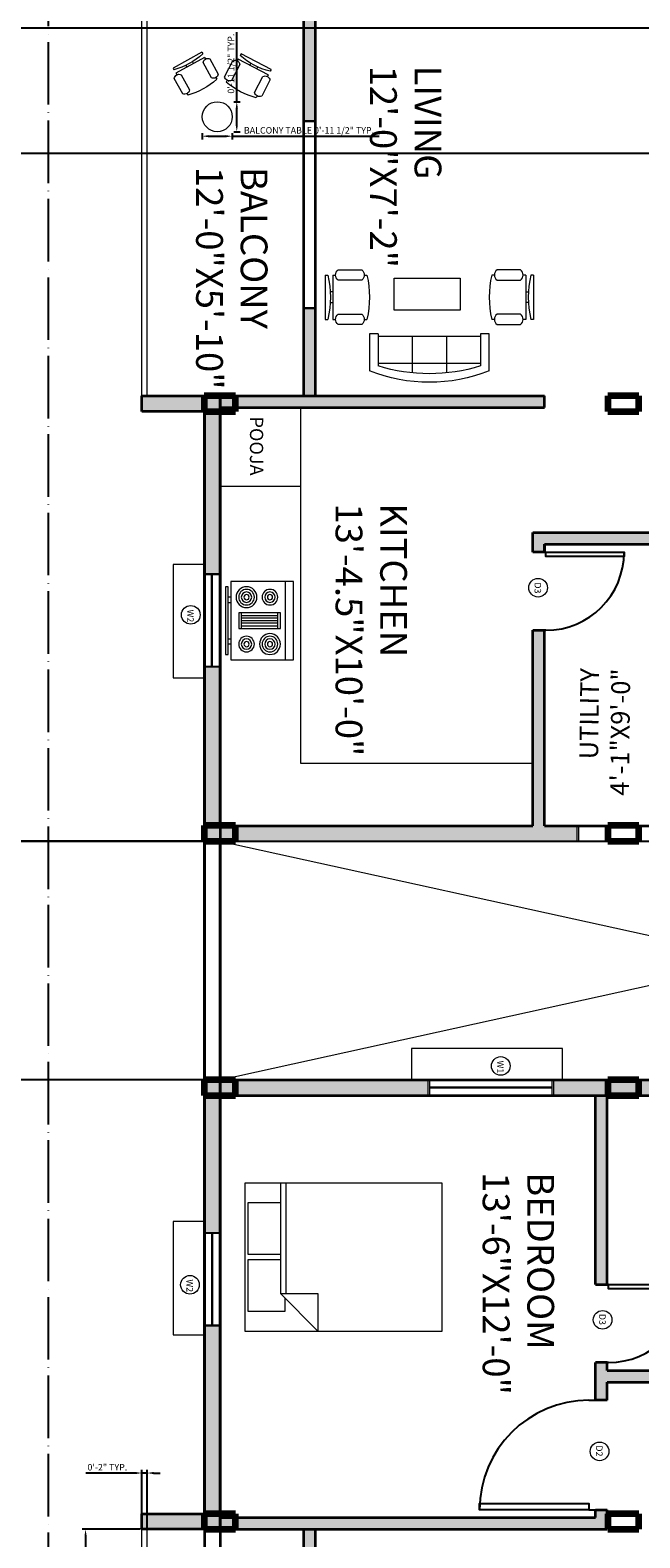
# Model space of a CAD drawing. Units: inches. Extents: x 7028582 to 7030319, y 63109697 to 63111305.
# Tile 8 of 18: x 7029168 to 7029402, y 63110278 to 63110857. Entities that reach past the tile are written whole.
import ezdxf

# ---------------------------------------------------------------- set-up
doc = ezdxf.new("R2010")
doc.units = ezdxf.units.IN
doc.linetypes.add('ACAD_ISO04W100', pattern=[30, 24, -3, 0, -3])
for name, color, linetype, lineweight in [('A-AREA-IDEN', 7, 'Continuous', 18), ('A-DOOR-IDEN', 20, 'Continuous', 13), ('A-EQPM', 9, 'Continuous', 18), ('A-FLOR-CASE', 9, 'Continuous', 18), ('A-FLOR-HRAL', 5, 'Continuous', 18), ('A-FLOR-OPEN', 7, 'Continuous', 13), ('A-GLAZ-IDEN', 20, 'Continuous', 13), ('A-WALL-PATT', 8, 'Continuous', 13), ('C-ANNO-DIMS', 7, 'Continuous', 18), ('C-PROP', 1, 'ACAD_ISO04W100', 25), ('doors', 20, 'Continuous', 25), ('furniture', 9, 'Continuous', 18), ('PILLARS', 220, 'Continuous', 100), ('walls', 6, 'Continuous', 35), ('WINDOW SHADOW', 9, 'Continuous', 13), ('windows', 5, 'Continuous', 18)]:
    doc.layers.add(name, color=color, linetype=linetype, lineweight=lineweight)
doc.styles.get("Standard").update_dxf_attribs({"font": 'arial.ttf'})
doc.dimstyles.new('ISO-25', dxfattribs={"dimtxt": 2.5, "dimasz": 2.5, "dimexe": 1.25, "dimexo": 0.625, "dimtad": 1, "dimlunit": 4, "dimtxsty": 'Standard', "dimcen": 2.5, "dimadec": 0, "dimazin": 0, "dimtfac": 1, "dimtmove": 0, "dimatfit": 3, "dimfxl": 1, "dimarcsym": 0})

# ---------------------------------------------------------------- blocks, each defined once
blk = doc.blocks.new('*U2')
for p, q in [((0, 0), (0, -5)), ((30, 0), (30, -5))]:
    blk.add_line(p, q)
blk.add_lwpolyline([(0, 0), (0, 30), (1.75, 30), (1.75, 0)], close=True)
blk.add_arc((0, 0), 30, 0, 90)
blk = doc.blocks.new('Range-Oven - 30 in top')
for p, q in [((0, -3), (30, -3)), ((12, -6), (18, -6)), ((13, -20), (13, -6)), ((14, -6), (14, -20)), ((15, -20), (15, -6)), ((16, -6), (16, -20)), ((17, -20), (17, -6)), ((18, -20), (12, -20)), ((6, -24), (6, -25)), ((8, -25), (8, -24)), ((22, -25), (22, -24)), ((24, -24), (24, -25))]:
    blk.add_line(p, q)
for points in [[(0, -24), (0, 0), (30, 0), (30, -24)], [(12, -21), (12, -5), (18, -5), (18, -21)], [(2, -26), (2, -25), (28, -25), (28, -26)]]:
    blk.add_lwpolyline(points, close=True)
for centre, radius in [((6, -9), 4), ((6, -9), 3), ((6, -9), 2), ((6, -9), 1), ((24, -9), 3), ((24, -9), 2), ((24, -9), 1), ((6, -18), 3), ((6, -18), 2), ((6, -18), 1), ((24, -18), 4), ((24, -18), 3), ((24, -18), 2), ((24, -18), 1)]:
    blk.add_circle(centre, radius)
blk = doc.blocks.new('Chair - Desk')
for p, q in [((-8.5, 0), (-8.5, -1)), ((-8.5, 0), (8.5, 0)), ((8.5, 0), (8.5, -1)), ((-10.5, -5), (-10.5, -14)), ((-8.5, -3), (-8.5, -4)), ((-8.5, -3), (8.5, -3)), ((-6.5, -14), (-6.5, -5)), ((-2, -3), (-2, -1.9355)), ((2, -1.9576), (2, -3)), ((6.5, -5), (6.5, -14)), ((8.5, -3), (8.5, -4)), ((10.5, -14), (10.5, -5)), ((-8.5, -15), (-8.5, -16)), ((8.5, -15), (8.5, -16))]:
    blk.add_line(p, q)
for centre, radius, start, end in [((-8.5, -6.5), 2.5, 36.8699, 143.1301), ((0, 34.625), 36.625, 256.5803, 283.4197), ((8.5, -6.5), 2.5, 36.8699, 143.1301), ((-8.5, -12.5), 2.5, 216.8699, 323.1301), ((0, 19.625), 36.625, 256.5803, 283.4197), ((8.5, -12.5), 2.5, 216.8699, 323.1301)]:
    blk.add_arc(centre, radius, start, end)
blk = doc.blocks.new('Sofa - Roundback 7 ft.')
for p, q in [((-12.00002, -32.4421), (-12.00003, -6.5971)), ((11.99997, -32.4421), (11.99998, -6.5971)), ((-36.000027, -34), (-36.000027, -11.4696)), ((-35.999844, -13.3819), (35.9998, -13.3819)), ((35.99998, -34), (35.99998, -11.4696)), ((-36.000027, -32.4421), (35.99998, -32.4421))]:
    blk.add_line(p, q)
for points in [[(-36.000027, -34), (-42.000027, -34), (-42.000027, -8)], [(41.99998, -8), (41.99998, -34), (35.99998, -34)]]:
    blk.add_lwpolyline(points)
for centre, radius, start, end in [((0, -114.25), 114.25, 68.43141, 111.5686), ((-0.00001, -127.1968), 121.1968, 72.72033, 107.2797)]:
    blk.add_arc(centre, radius, start, end)
blk = doc.blocks.new('Bed - Queen')
for p, q in [((0, -80.00003), (0, 0)), ((0, 0), (59.99999, 0)), ((59.99999, 0), (59.99999, -80.00003)), ((7.99999, -1.2), (28.79998, -1.2)), ((7.99999, -14.4), (7.99999, -1.2)), ((28.79998, -1.2), (28.79998, -14.4)), ((31.19999, -1.2), (51.99999, -1.2)), ((31.19999, -14.4), (31.19999, -1.2)), ((51.99999, -1.2), (51.99999, -16.4)), ((0, -14.4), (44.8, -14.4)), ((44.8, -16.8), (0, -16.8)), ((59.99999, -29.6), (44.8, -14.4)), ((44.8, -14.4), (44.8, -29.6)), ((51.99999, -16.4), (46.79936, -16.4)), ((44.8, -29.6), (59.99999, -29.6)), ((59.99999, -80.00003), (0, -80.00003))]:
    blk.add_line(p, q)
blk = doc.blocks.new('WIN-SASH-36')
for p, q in [((0, 36.05), (0, 0)), ((6, 35.55), (0, 35.55)), ((2.8, 35.55), (2.8, 0.5)), ((3.2, 35.55), (3.2, 0.5)), ((6, 0), (6, 36.05)), ((0, 0.5), (6, 0.5))]:
    blk.add_line(p, q)
blk = doc.blocks.new('WIN-SASH-24-FRAME')
for p, q in [((24.05, 6), (0, 6)), ((0.5, 6), (0.5, 0)), ((23.55, 0), (23.55, 6)), ((0, 0), (24.05, 0))]:
    blk.add_line(p, q)
blk = doc.blocks.new('WIN-SASH-48')
for p, q in [((48.05, 6), (0, 6)), ((0.5, 6), (0.5, 0)), ((47.55, 0), (47.55, 6)), ((47.55, 3.2), (0.5, 3.2)), ((47.55, 2.8), (0.5, 2.8)), ((0, 0), (48.05, 0))]:
    blk.add_line(p, q)
blk = doc.blocks.new('WIN-SASH-BALCONY')
for p, q in [((0.13, 72.09), (0.13, 36.05)), ((4.63, 71.71), (0.13, 71.71)), ((4.63, 36.05), (4.63, 72.09)), ((0, 0.02), (0.13, 36.05)), ((0.13, 35.68), (0.13, 35.68)), ((4.63, 36.04), (4.5, 0)), ((4.5, 0.37), (0, 0.39))]:
    blk.add_line(p, q)
blk = doc.blocks.new('WINDOW-SHADE-SIDE-44')
for p, q in [((12, 43.55), (0, 43.55)), ((12, 0), (12, 43.55)), ((0, 0), (12, 0))]:
    blk.add_line(p, q)
blk = doc.blocks.new('WINDOW-SHADE-HEAD-58')
for p, q in [((57.96, 12), (0, 12)), ((0, 12), (0, 0)), ((57.96, 0), (57.96, 12))]:
    blk.add_line(p, q)
blk = doc.blocks.new('KITCHEN-COUNTER')
for p, q in [((89.09, 136.54), (89.09, 16.65)), ((120, 106.35), (89.09, 106.35)), ((89.09, 16.65), (89.09, 0)), ((89.09, 0), (0, 0))]:
    blk.add_line(p, q)
blk = doc.blocks.new('COLUMN-RECT-PROFILE')
for p, q in [((11.91, 6), (0, 6)), ((0, 6), (0, 0)), ((11.91, 0), (11.91, 6)), ((0, 0), (11.91, 0))]:
    blk.add_line(p, q)
blk = doc.blocks.new('BALCONY-GUARD-12FT')
for p, q in [((0, 144), (0, 0)), ((2, 144), (2, 0))]:
    blk.add_line(p, q)
blk = doc.blocks.new('TABLE-COFFEE-RECT')
blk.add_lwpolyline([(25.34, 12.34), (0, 12.34), (0, 0), (25.34, 0)], close=True)
blk = doc.blocks.new('TAG-D3-MT-L')
blk.add_circle((3.58, 3.58), 3.58)
at = {"insert": (2.23, 5.6), "char_height": 2.5, "attachment_point": 7, "rotation": 270}
blk.add_mtext_dynamic_manual_height_columns('D3', width=2.5021, gutter_width=12.5, heights=[0], dxfattribs=at)
blk = doc.blocks.new('TAG-W2-MT-L')
blk.add_circle((3.58, 3.58), 3.58)
at = {"insert": (2.23, 5.6), "char_height": 2.5, "attachment_point": 7, "rotation": 270}
blk.add_mtext_dynamic_manual_height_columns('W2', width=2.5021, gutter_width=12.5, heights=[0], dxfattribs=at)
blk = doc.blocks.new('TAG-D2-ST-L')
blk.add_circle((3.58, 3.58), 3.58)
blk.add_text('D2', height=2.5, rotation=270).set_placement((2.23, 5.87))
blk = doc.blocks.new('TAG-D3-ST-L')
blk.add_circle((3.58, 3.58), 3.58)
blk.add_text('D3', height=2.5, rotation=270).set_placement((2.27, 5.87))
blk = doc.blocks.new('TAG-W1-ST-L')
blk.add_circle((3.58, 3.58), 3.58)
blk.add_text('W1', height=2.5, rotation=270).set_placement((2.23, 5.64))
blk = doc.blocks.new('TAG-W2-ST-L')
blk.add_circle((3.58, 3.58), 3.58)
blk.add_text('W2', height=2.5, rotation=270).set_placement((2.23, 5.64))
blk = doc.blocks.new('TABLE-BALCONY-ROUND')
blk.add_circle((5.75, 5.75), 5.75)
blk = doc.blocks.new('*D87')
at = {"layer": 'C-ANNO-DIMS', "color": 0, "lineweight": -2, "transparency": 16777216}
for p, q in [((7029210.08, 63110281.56), (7029187.86, 63110281.56)), ((7029189.11, 63110279.06), (7029189.11, 63110140.06)), ((7029210.08, 63110137.56), (7029187.86, 63110137.56))]:
    blk.add_line(p, q, dxfattribs=at)
at = {"layer": 'C-ANNO-DIMS', "color": 0, "lineweight": 100, "transparency": 16777216}
for points in [[(7029188.69, 63110279.06), (7029189.52, 63110279.06), (7029189.11, 63110281.56)], [(7029188.69, 63110140.06), (7029189.52, 63110140.06), (7029189.11, 63110137.56)]]:
    blk.add_solid(points, dxfattribs=at)
at = {"layer": 'Defpoints', "color": 0, "lineweight": 100, "transparency": 16777216}
for p in [(7029210.71, 63110281.56), (7029189.11, 63110137.56), (7029210.71, 63110137.56)]:
    blk.add_point(p, dxfattribs=at)
at = {"layer": 'C-ANNO-DIMS', "color": 0, "transparency": 16777216, "insert": (7029187.19, 63110209.56), "char_height": 2.5, "attachment_point": 5, "rotation": 90}
blk.add_mtext('GUARD 12\'-0" TYP.', dxfattribs=at)
blk = doc.blocks.new('*D88')
at = {"layer": 'C-ANNO-DIMS', "color": 0, "lineweight": -2, "transparency": 16777216}
for p, q in [((7029210.71, 63110282.18), (7029210.71, 63110304.41)), ((7029212.71, 63110282.18), (7029212.71, 63110304.41)), ((7029208.21, 63110303.16), (7029189.22, 63110303.16)), ((7029212.71, 63110303.16), (7029210.71, 63110303.16)), ((7029215.21, 63110303.16), (7029217.71, 63110303.16))]:
    blk.add_line(p, q, dxfattribs=at)
at = {"layer": 'C-ANNO-DIMS', "color": 0, "lineweight": 100, "transparency": 16777216}
for points in [[(7029208.21, 63110303.57), (7029208.21, 63110302.74), (7029210.71, 63110303.16)], [(7029215.21, 63110303.57), (7029215.21, 63110302.74), (7029212.71, 63110303.16)]]:
    blk.add_solid(points, dxfattribs=at)
at = {"layer": 'Defpoints', "color": 0, "lineweight": 100, "transparency": 16777216}
for p in [(7029210.71, 63110303.16), (7029210.71, 63110281.56), (7029212.71, 63110281.56)]:
    blk.add_point(p, dxfattribs=at)
at = {"layer": 'C-ANNO-DIMS', "color": 0, "transparency": 16777216, "insert": (7029197.46, 63110305.06), "char_height": 2.5, "attachment_point": 5}
blk.add_mtext('0\'-2" TYP.', dxfattribs=at)
blk = doc.blocks.new('*D89')
at = {"layer": 'C-ANNO-DIMS', "color": 0, "lineweight": -2, "transparency": 16777216}
for p, q in [((7029233.89, 63110817.25), (7029233.89, 63110814.9)), ((7029236.39, 63110816.15), (7029242.89, 63110816.15)), ((7029245.39, 63110817.25), (7029245.39, 63110814.9)), ((7029245.39, 63110816.15), (7029301.73, 63110816.15))]:
    blk.add_line(p, q, dxfattribs=at)
at = {"layer": 'C-ANNO-DIMS', "color": 0, "lineweight": 100, "transparency": 16777216}
for points in [[(7029236.39, 63110816.57), (7029236.39, 63110815.73), (7029233.89, 63110816.15)], [(7029242.89, 63110816.57), (7029242.89, 63110815.73), (7029245.39, 63110816.15)]]:
    blk.add_solid(points, dxfattribs=at)
at = {"layer": 'Defpoints', "color": 0, "lineweight": 100, "transparency": 16777216}
for p in [(7029233.89, 63110817.87), (7029245.39, 63110817.87), (7029245.39, 63110816.15)]:
    blk.add_point(p, dxfattribs=at)
at = {"layer": 'C-ANNO-DIMS', "color": 0, "transparency": 16777216, "insert": (7029274.81, 63110818.07), "char_height": 2.5, "attachment_point": 5}
blk.add_mtext('BALCONY TABLE 0\'-11 1/2" TYP.', dxfattribs=at)
blk = doc.blocks.new('*D90')
at = {"layer": 'C-ANNO-DIMS', "color": 0, "lineweight": -2, "transparency": 16777216}
for p, q in [((7029247.11, 63110829.37), (7029247.11, 63110856.13)), ((7029246.01, 63110829.37), (7029248.36, 63110829.37)), ((7029247.11, 63110820.37), (7029247.11, 63110826.87)), ((7029246.01, 63110817.87), (7029248.36, 63110817.87))]:
    blk.add_line(p, q, dxfattribs=at)
at = {"layer": 'C-ANNO-DIMS', "color": 0, "lineweight": 100, "transparency": 16777216}
for points in [[(7029246.7, 63110826.87), (7029247.53, 63110826.87), (7029247.11, 63110829.37)], [(7029246.7, 63110820.37), (7029247.53, 63110820.37), (7029247.11, 63110817.87)]]:
    blk.add_solid(points, dxfattribs=at)
at = {"layer": 'Defpoints', "color": 0, "lineweight": 100, "transparency": 16777216}
for p in [(7029245.39, 63110829.37), (7029247.11, 63110829.37), (7029245.39, 63110817.87)]:
    blk.add_point(p, dxfattribs=at)
at = {"layer": 'C-ANNO-DIMS', "color": 0, "transparency": 16777216, "insert": (7029245.19, 63110844), "char_height": 2.5, "attachment_point": 5, "rotation": 90}
blk.add_mtext('0\'-11 1/2" TYP.', dxfattribs=at)
blk = doc.blocks.new('*D100')
at = {"layer": 'C-ANNO-DIMS', "color": 0, "lineweight": -2, "transparency": 16777216}
for p, q in [((7029234.08, 63111033.06), (7028586.23, 63111033.06)), ((7028587.48, 63109969.06), (7028587.48, 63111030.56)), ((7029234.08, 63109966.56), (7028586.23, 63109966.56))]:
    blk.add_line(p, q, dxfattribs=at)
at = {"layer": 'C-ANNO-DIMS', "color": 0, "lineweight": 100, "transparency": 16777216}
for points in [[(7028587.06, 63111030.56), (7028587.89, 63111030.56), (7028587.48, 63111033.06)], [(7028587.06, 63109969.06), (7028587.89, 63109969.06), (7028587.48, 63109966.56)]]:
    blk.add_solid(points, dxfattribs=at)
at = {"layer": 'Defpoints', "color": 0, "lineweight": 100, "transparency": 16777216}
for p in [(7028587.48, 63111033.06), (7029234.71, 63111033.06), (7029234.71, 63109966.56)]:
    blk.add_point(p, dxfattribs=at)
at = {"layer": 'C-ANNO-DIMS', "color": 0, "transparency": 16777216, "insert": (7028585.56, 63110499.81), "char_height": 2.5, "attachment_point": 5, "rotation": 90}
blk.add_mtext('88\'-10 1/2"', dxfattribs=at)
blk = doc.blocks.new('*D103')
at = {"layer": 'C-ANNO-DIMS', "color": 0, "lineweight": -2, "transparency": 16777216}
for p, q in [((7029234.03, 63110545.61), (7028586.23, 63110545.61)), ((7028587.48, 63110456.56), (7028587.48, 63110543.11)), ((7029234.08, 63110454.06), (7028586.23, 63110454.06))]:
    blk.add_line(p, q, dxfattribs=at)
at = {"layer": 'C-ANNO-DIMS', "color": 0, "lineweight": 100, "transparency": 16777216}
for points in [[(7028587.06, 63110543.11), (7028587.89, 63110543.11), (7028587.48, 63110545.61)], [(7028587.06, 63110456.56), (7028587.89, 63110456.56), (7028587.48, 63110454.06)]]:
    blk.add_solid(points, dxfattribs=at)
at = {"layer": 'Defpoints', "color": 0, "lineweight": 100, "transparency": 16777216}
for p in [(7028587.48, 63110545.61), (7029234.66, 63110545.61), (7029234.71, 63110454.06)]:
    blk.add_point(p, dxfattribs=at)
at = {"layer": 'C-ANNO-DIMS', "color": 0, "transparency": 16777216, "insert": (7028585.56, 63110499.83), "char_height": 2.5, "attachment_point": 5, "rotation": 90}
blk.add_mtext('7\'-7 1/2"', dxfattribs=at)
blk = doc.blocks.new('*D104')
at = {"layer": 'C-ANNO-DIMS', "color": 0, "lineweight": -2, "transparency": 16777216}
for p, q in [((7029747.58, 63110857.56), (7028586.23, 63110857.56)), ((7028587.48, 63110812.06), (7028587.48, 63110855.06)), ((7029747.58, 63110809.56), (7028586.23, 63110809.56))]:
    blk.add_line(p, q, dxfattribs=at)
at = {"layer": 'C-ANNO-DIMS', "color": 0, "lineweight": 100, "transparency": 16777216}
for points in [[(7028587.06, 63110855.06), (7028587.89, 63110855.06), (7028587.48, 63110857.56)], [(7028587.06, 63110812.06), (7028587.89, 63110812.06), (7028587.48, 63110809.56)]]:
    blk.add_solid(points, dxfattribs=at)
at = {"layer": 'Defpoints', "color": 0, "lineweight": 100, "transparency": 16777216}
for p in [(7028587.48, 63110857.56), (7029748.21, 63110857.56), (7029748.21, 63110809.56)]:
    blk.add_point(p, dxfattribs=at)
at = {"layer": 'C-ANNO-DIMS', "color": 0, "transparency": 16777216, "insert": (7028585.57, 63110833.56), "char_height": 2.5, "attachment_point": 5, "rotation": 90}
blk.add_mtext('4\'-0"', dxfattribs=at)
blk = doc.blocks.new('*D112')
at = {"layer": 'C-ANNO-DIMS', "color": 0, "lineweight": -2, "transparency": 16777216}
for p, q in [((7029747.58, 63111033.06), (7028586.23, 63111033.06)), ((7028587.48, 63111030.56), (7028587.48, 63110548.06)), ((7029747.58, 63110545.56), (7028586.23, 63110545.56))]:
    blk.add_line(p, q, dxfattribs=at)
at = {"layer": 'C-ANNO-DIMS', "color": 0, "lineweight": 100, "transparency": 16777216}
for points in [[(7028587.06, 63111030.56), (7028587.89, 63111030.56), (7028587.48, 63111033.06)], [(7028587.06, 63110548.06), (7028587.89, 63110548.06), (7028587.48, 63110545.56)]]:
    blk.add_solid(points, dxfattribs=at)
at = {"layer": 'Defpoints', "color": 0, "lineweight": 100, "transparency": 16777216}
for p in [(7029748.21, 63111033.06), (7028587.48, 63110545.56), (7029748.21, 63110545.56)]:
    blk.add_point(p, dxfattribs=at)
at = {"layer": 'C-ANNO-DIMS', "color": 0, "transparency": 16777216, "insert": (7028585.56, 63110789.31), "char_height": 2.5, "attachment_point": 5, "rotation": 90}
blk.add_mtext('40\'-7 1/2"', dxfattribs=at)

msp = doc.modelspace()

# ---------------------------------------------------------------- hatches: boundary and pattern name
at = {"layer": 'A-WALL-PATT'}
h = msp.add_hatch(color=256, dxfattribs=at)
h.dxf.hatch_style = 1
h.paths.add_polyline_path([(7029272.705, 63110860.557), (7029277.205, 63110860.557), (7029277.205, 63110822.163), (7029272.705, 63110822.163)])
h = msp.add_hatch(color=256, dxfattribs=at)
h.dxf.hatch_style = 1
h.paths.add_polyline_path([(7029272.705, 63110716.557), (7029277.205, 63110716.557), (7029277.205, 63110750.09), (7029272.705, 63110750.074)])
h = msp.add_hatch(color=256, dxfattribs=at)
h.dxf.hatch_style = 1
h.paths.add_polyline_path([(7029210.705, 63110716.557), (7029234.705, 63110716.557), (7029234.705, 63110710.557), (7029210.705, 63110710.557)])
h = msp.add_hatch(color=256, dxfattribs=at)
h.dxf.hatch_style = 1
h.paths.add_polyline_path([(7029234.705, 63110716.557), (7029240.705, 63110716.557), (7029240.705, 63110648.386), (7029234.705, 63110648.386)])
h = msp.add_hatch(color=256, dxfattribs=at)
h.dxf.hatch_style = 1
h.paths.add_polyline_path([(7029240.705, 63110716.557), (7029240.705, 63110712.057), (7029365.205, 63110712.057), (7029365.205, 63110716.557)])
h = msp.add_hatch(color=256, dxfattribs=at)
h.dxf.hatch_style = 1
h.paths.add_polyline_path([(7029414.205, 63110659.557), (7029414.205, 63110664.057), (7029360.705, 63110664.057), (7029360.705, 63110656.557), (7029365.205, 63110656.557), (7029365.205, 63110659.557)])
h = msp.add_hatch(color=256, dxfattribs=at)
h.dxf.hatch_style = 1
h.paths.add_polyline_path([(7029234.705, 63110612.338), (7029240.705, 63110612.338), (7029240.705, 63110551.557), (7029360.705, 63110551.557), (7029360.705, 63110626.557), (7029365.205, 63110626.557), (7029365.205, 63110551.557), (7029377.666, 63110551.557), (7029377.666, 63110545.557), (7029234.705, 63110545.557)])
h = msp.add_hatch(color=256, dxfattribs=at)
h.dxf.hatch_style = 1
h.paths.add_polyline_path([(7029234.705, 63110454.057), (7029320.549, 63110454.057), (7029320.549, 63110448.057), (7029240.705, 63110448.057), (7029240.705, 63110395.515), (7029234.705, 63110395.515)])
h = msp.add_hatch(color=256, dxfattribs=at)
h.dxf.hatch_style = 1
h.paths.add_polyline_path([(7029368.597, 63110454.057), (7029405.832, 63110454.057), (7029405.832, 63110448.057), (7029368.597, 63110448.057)])
h.paths.add_polyline_path([(7029384.705, 63110448.057), (7029389.205, 63110448.057), (7029389.205, 63110375.557), (7029384.705, 63110375.557)], flags=0)
h = msp.add_hatch(color=256, dxfattribs=at)
h.dxf.hatch_style = 1
h.paths.add_polyline_path([(7029384.705, 63110448.057), (7029389.205, 63110448.057), (7029389.205, 63110375.557), (7029384.705, 63110375.557)], flags=0)
h.paths.add_polyline_path([(7029384.705, 63110345.557), (7029389.205, 63110345.557), (7029389.205, 63110342.557), (7029444.205, 63110342.557), (7029444.205, 63110448.057), (7029448.705, 63110448.057), (7029448.705, 63110342.557), (7029469.705, 63110342.557), (7029469.705, 63110338.057), (7029448.705, 63110338.057), (7029448.705, 63110286.057), (7029526.726, 63110286.057), (7029526.726, 63110281.557), (7029444.205, 63110281.557), (7029444.205, 63110338.057), (7029389.205, 63110338.057), (7029389.205, 63110331.057), (7029384.705, 63110331.057)])
h = msp.add_hatch(color=256, dxfattribs=at)
h.dxf.hatch_style = 1
h.paths.add_polyline_path([(7029389.205, 63110448.057), (7029384.705, 63110448.057), (7029384.705, 63110375.557), (7029389.205, 63110375.557)])
h = msp.add_hatch(color=256, dxfattribs=at)
h.dxf.hatch_style = 1
h.paths.add_polyline_path([(7029234.705, 63110281.557), (7029240.705, 63110281.557), (7029240.705, 63110359.466), (7029234.705, 63110359.466)])
h = msp.add_hatch(color=256, dxfattribs=at)
h.dxf.hatch_style = 1
h.paths.add_polyline_path([(7029210.705, 63110287.557), (7029234.705, 63110287.557), (7029234.705, 63110281.557), (7029210.705, 63110281.557)])
h = msp.add_hatch(color=256, dxfattribs=at)
h.dxf.hatch_style = 1
h.paths.add_polyline_path([(7029240.705, 63110286.057), (7029384.705, 63110286.057), (7029384.705, 63110289.057), (7029389.205, 63110289.057), (7029389.205, 63110281.557), (7029240.705, 63110281.557)])
h = msp.add_hatch(color=256, dxfattribs=at)
h.dxf.hatch_style = 1
h.paths.add_polyline_path([(7029272.705, 63110281.557), (7029277.205, 63110281.557), (7029277.205, 63110243.163), (7029272.705, 63110243.163)])

# ---------------------------------------------------------------- linework, layer by layer
at = {"layer": 'A-FLOR-OPEN'}
for p, q in [((7029656.205, 63110454.057), (7029240.705, 63110545.557)), ((7029240.705, 63110454.057), (7029656.205, 63110545.557))]:
    msp.add_line(p, q, dxfattribs=at)
at = {"layer": 'C-PROP'}
msp.add_line((7029174.705, 63111093.057), (7029174.705, 63109906.557), dxfattribs=at)
at = {"layer": 'walls'}
for p, q in [((7029272.705, 63110860.557), (7029272.705, 63110716.557)), ((7029277.205, 63110860.557), (7029277.205, 63110716.557)), ((7029210.705, 63110710.557), (7029210.705, 63110716.557)), ((7029210.705, 63110716.557), (7029234.705, 63110716.557)), ((7029234.705, 63110281.557), (7029234.705, 63110716.557)), ((7029234.705, 63110716.557), (7029365.205, 63110716.557)), ((7029234.705, 63110716.557), (7029234.705, 63109966.557)), ((7029240.705, 63110551.557), (7029240.705, 63110716.557)), ((7029240.705, 63110716.557), (7029240.705, 63109972.557)), ((7029365.205, 63110712.057), (7029365.205, 63110716.557)), ((7029234.705, 63110710.557), (7029210.705, 63110710.557)), ((7029240.705, 63110712.057), (7029365.205, 63110712.057)), ((7029360.705, 63110656.557), (7029360.705, 63110664.057)), ((7029360.705, 63110664.057), (7029445.705, 63110664.057)), ((7029365.205, 63110656.557), (7029360.705, 63110656.557)), ((7029365.205, 63110656.557), (7029365.205, 63110659.557)), ((7029365.205, 63110659.557), (7029445.705, 63110659.557)), ((7029365.205, 63110659.557), (7029365.205, 63110656.557)), ((7029360.705, 63110551.557), (7029360.705, 63110626.557)), ((7029360.705, 63110626.557), (7029365.205, 63110626.557)), ((7029365.205, 63110551.557), (7029365.205, 63110626.557)), ((7029240.705, 63110551.557), (7029360.705, 63110551.557)), ((7029365.205, 63110551.557), (7029414.205, 63110551.557)), ((7029240.705, 63110281.557), (7029240.705, 63110545.557)), ((7029240.705, 63110454.057), (7029234.705, 63110454.057)), ((7029234.705, 63110281.557), (7029234.705, 63110454.057)), ((7029234.705, 63110454.057), (7029585.16, 63110454.057)), ((7029240.705, 63110281.557), (7029240.705, 63110448.057)), ((7029240.705, 63110448.057), (7029662.205, 63110448.057)), ((7029384.705, 63110375.557), (7029384.705, 63110448.057)), ((7029389.205, 63110375.557), (7029389.205, 63110448.057)), ((7029384.705, 63110375.557), (7029389.205, 63110375.557)), ((7029384.705, 63110331.057), (7029384.705, 63110345.557)), ((7029389.205, 63110345.557), (7029384.705, 63110345.557)), ((7029389.205, 63110342.557), (7029389.205, 63110345.557)), ((7029389.205, 63110342.557), (7029389.205, 63110345.557)), ((7029389.205, 63110342.557), (7029444.205, 63110342.557)), ((7029389.205, 63110331.057), (7029389.205, 63110338.057)), ((7029389.205, 63110338.057), (7029444.205, 63110338.057)), ((7029389.205, 63110331.057), (7029384.705, 63110331.057)), ((7029210.705, 63110281.557), (7029210.705, 63110287.557)), ((7029210.705, 63110287.557), (7029234.705, 63110287.557)), ((7029240.705, 63110286.057), (7029384.705, 63110286.057)), ((7029384.705, 63110286.057), (7029384.705, 63110289.057)), ((7029384.705, 63110286.057), (7029384.705, 63110289.057)), ((7029384.705, 63110289.057), (7029389.205, 63110289.057)), ((7029389.205, 63110281.557), (7029389.205, 63110289.057)), ((7029234.705, 63110281.557), (7029210.705, 63110281.557)), ((7029234.705, 63110281.557), (7029389.205, 63110281.557)), ((7029272.705, 63110281.557), (7029272.705, 63110137.557)), ((7029277.205, 63110281.557), (7029277.205, 63110137.557))]:
    msp.add_line(p, q, dxfattribs=at)
at = {"layer": 'windows'}
for p, q in [((7029272.705, 63110822.163), (7029277.205, 63110822.163)), ((7029272.834, 63110750.074), (7029277.334, 63110750.09)), ((7029234.512, 63110648.386), (7029240.512, 63110648.386)), ((7029240.512, 63110612.338), (7029234.512, 63110612.338)), ((7029377.666, 63110545.557), (7029377.666, 63110551.557)), ((7029320.549, 63110448.057), (7029320.549, 63110454.057)), ((7029368.597, 63110454.057), (7029368.597, 63110448.057)), ((7029234.635, 63110395.515), (7029240.635, 63110395.515)), ((7029240.635, 63110359.466), (7029234.635, 63110359.466))]:
    msp.add_line(p, q, dxfattribs=at)

# ---------------------------------------------------------------- block references
at = {"layer": 'A-DOOR-IDEN'}
for name, p in [('TAG-D3-MT-L', (7029359.103, 63110639.309)), ('TAG-D3-ST-L', (7029383.855, 63110358.359)), ('TAG-D2-ST-L', (7029382.689, 63110307.879))]:
    msp.add_blockref(name, p, dxfattribs=at)
at = {"layer": 'A-EQPM', "xscale": -1, "rotation": 270}
msp.add_blockref('Range-Oven - 30 in top', (7029268.844, 63110615.257), dxfattribs=at)
at = {"layer": 'A-FLOR-CASE', "extrusion": (0, 0, -1), "zscale": -1}
msp.add_blockref('KITCHEN-COUNTER', (-7029360.705, 63110575.518), dxfattribs=at)
at = {"layer": 'A-FLOR-HRAL', "rotation": 180}
for p in [(7029212.705, 63110860.557), (7029212.705, 63110281.557)]:
    msp.add_blockref('BALCONY-GUARD-12FT', p, dxfattribs=at)
at = {"layer": 'A-GLAZ-IDEN'}
for name, p in [('TAG-W2-MT-L', (7029225.884, 63110628.907)), ('TAG-W1-ST-L', (7029344.79, 63110455.779)), ('TAG-W2-ST-L', (7029225.585, 63110371.827))]:
    msp.add_blockref(name, p, dxfattribs=at)
at = {"layer": 'doors', "rotation": 270}
for p in [(7029365.705, 63110656.557), (7029389.705, 63110375.557)]:
    msp.add_blockref('*U2', p, dxfattribs=at)
at = {"layer": 'doors', "xscale": 1.399999999999999, "yscale": 1.399999999999999, "zscale": 1.399999999999999, "rotation": 90.00000000000003}
msp.add_blockref('*U2', (7029382.205, 63110289.057), dxfattribs=at)
at = {"layer": 'furniture'}
for name, p, xscale, yscale, zscale, rotation in [('Chair - Desk', (7029228.177, 63110845.309), -0.740937522274531, 0.740937522274531, 0.740937522274531, 28.89971253738977), ('Chair - Desk', (7029254.497, 63110844.758), -0.7643373636972337, 0.7643373636972337, 0.7643373636972337, 332.4708086599736), ('Sofa - Roundback 7 ft.', (7029320.972, 63110721.72), -0.5455524879488546, 0.5455524879488546, 0.5455524879488546, 180), ('Bed - Queen', (7029250.204, 63110414.435), -0.9464141645025947, 0.9464141645025947, 0.9464141645025947, 90)]:
    msp.add_blockref(name, p, dxfattribs=dict(at, xscale=xscale, yscale=yscale, zscale=zscale, rotation=rotation))
msp.add_blockref('TABLE-BALCONY-ROUND', (7029233.889, 63110817.874), dxfattribs=at)
at = {"layer": 'furniture', "xscale": -1, "rotation": 90}
msp.add_blockref('Chair - Desk', (7029281.016, 63110754.367), dxfattribs=at)
at = {"layer": 'furniture', "extrusion": (0, 0, -1), "zscale": -1}
msp.add_blockref('TABLE-COFFEE-RECT', (-7029332.859, 63110749.363), dxfattribs=at)
at = {"layer": 'furniture', "rotation": 270}
msp.add_blockref('Chair - Desk', (7029360.929, 63110754.367), dxfattribs=at)
at = {"layer": 'PILLARS'}
for p in [(7029234.659, 63110710.557), (7029389.44, 63110710.557), (7029234.659, 63110545.607), (7029389.44, 63110545.607), (7029234.659, 63110448.057), (7029389.44, 63110448.057), (7029234.659, 63110281.557), (7029389.44, 63110281.557)]:
    msp.add_blockref('COLUMN-RECT-PROFILE', p, dxfattribs=at)
at = {"layer": 'WINDOW SHADOW', "rotation": 180}
for p in [(7029234.706, 63110651.829), (7029234.706, 63110399.719)]:
    msp.add_blockref('WINDOW-SHADE-SIDE-44', p, dxfattribs=at)
at = {"layer": 'WINDOW SHADOW'}
msp.add_blockref('WINDOW-SHADE-HEAD-58', (7029314.122, 63110454.057), dxfattribs=at)
at = {"layer": 'windows', "extrusion": (0, 0, -1), "zscale": -1}
msp.add_blockref('WIN-SASH-BALCONY', (-7029277.334, 63110750.074), dxfattribs=at)
at = {"layer": 'windows'}
for name, p in [('WIN-SASH-36', (7029234.512, 63110612.338)), ('WIN-SASH-24-FRAME', (7029377.666, 63110545.557)), ('WIN-SASH-48', (7029320.549, 63110448.057)), ('WIN-SASH-36', (7029234.635, 63110359.466))]:
    msp.add_blockref(name, p, dxfattribs=at)

# ---------------------------------------------------------------- texts
at = {"layer": 'A-AREA-IDEN'}
for s, width, gutter_width, insert, char_height, attachment_point, rotation in [('LIVING\\P12\'-0"X7\'-2"', 82.04322, 51.315, (7029298.218, 63110843.231), 10.26307, 7, 270), ('BALCONY\\P12\'-0"X5\'-10"', 82.04322, 51.315, (7029231.516, 63110804.354), 10.26307, 7, 270), ('POOJA', 15.69653, 25.463, (7029252.151, 63110708.57), 5.0926, 7, 270), ('KITCHEN\\P13\'-4.5"X10\'-0"', 82.04322, 51.315, (7029285.025, 63110675.255), 10.26307, 7, 270), ('UTILITY\\P4\'-1"X9\'-0"', 42.97461, 35.821, (7029378.929, 63110612.048), 7.16426, 3, 89.353601), ('BEDROOM\\P13\'-6"X12\'-0"', 82.04322, 51.315, (7029341.455, 63110418.575), 10.26307, 7, 270)]:
    msp.add_mtext_dynamic_manual_height_columns(s, width=width, gutter_width=gutter_width, heights=[0], dxfattribs=dict(at, insert=insert, char_height=char_height, attachment_point=attachment_point, rotation=rotation))

# ---------------------------------------------------------------- dimensions: what is measured, and where the dimension line sits
at = {"layer": 'C-ANNO-DIMS'}
for base, p1, p2, picture, middle in [((7028587.475, 63111033.057), (7029234.705, 63109966.557), (7029234.705, 63111033.057), '*D100', (7028585.558, 63110499.807)), ((7028587.475, 63110545.557), (7029748.205, 63111033.057), (7029748.205, 63110545.557), '*D112', (7028585.558, 63110789.307)), ((7028587.475, 63110857.557), (7029748.205, 63110809.557), (7029748.205, 63110857.557), '*D104', (7028585.574, 63110833.557)), ((7028587.4754, 63110545.6071), (7029234.7053, 63110454.0567), (7029234.6592, 63110545.6071), '*D103', (7028585.5578, 63110499.8319))]:
    dim = msp.add_linear_dim(base=base, p1=p1, p2=p2, angle=90, dimstyle='ISO-25', override={"dimdec": 1, "dimlfac": 1, "dimrnd": 0, "dimzin": 1, "dimdsep": 46, "dimlunit": 4, "dimfrac": 2}, dxfattribs=at)
    dim.commit()
    dim.dimension.update_dxf_attribs({"geometry": picture, "text_midpoint": middle})
for base, p1, p2, angle, text, picture, middle in [((7029247.112, 63110829.372), (7029245.387, 63110817.874), (7029245.387, 63110829.372), 90, '<> TYP.', '*D90', (7029245.195, 63110844.001)), ((7029210.705, 63110303.157), (7029212.705, 63110281.557), (7029210.705, 63110281.557), 180, '<> TYP.', '*D88', (7029197.461, 63110305.058)), ((7029189.105, 63110137.557), (7029210.705, 63110281.557), (7029210.705, 63110137.557), 270, 'GUARD <> TYP.', '*D87', (7029187.188, 63110209.557))]:
    dim = msp.add_linear_dim(base=base, p1=p1, p2=p2, angle=angle, text=text, dimstyle='ISO-25', override={"dimdec": 1, "dimlfac": 1, "dimrnd": 0, "dimzin": 1, "dimdsep": 46, "dimlunit": 4, "dimfrac": 2}, dxfattribs=at)
    dim.commit()
    dim.dimension.update_dxf_attribs({"geometry": picture, "text_midpoint": middle})
dim = msp.add_linear_dim(base=(7029245.387, 63110816.149), p1=(7029233.889, 63110817.874), p2=(7029245.387, 63110817.874), text='BALCONY TABLE <> TYP.', dimstyle='ISO-25', override={"dimdec": 1, "dimlfac": 1, "dimrnd": 0, "dimzin": 1, "dimdsep": 46, "dimlunit": 4, "dimfrac": 2}, dxfattribs=at)
dim.commit()
dim.dimension.update_dxf_attribs({"geometry": '*D89', "text_midpoint": (7029274.808, 63110818.068)})

doc.saveas('drawing.dxf')
